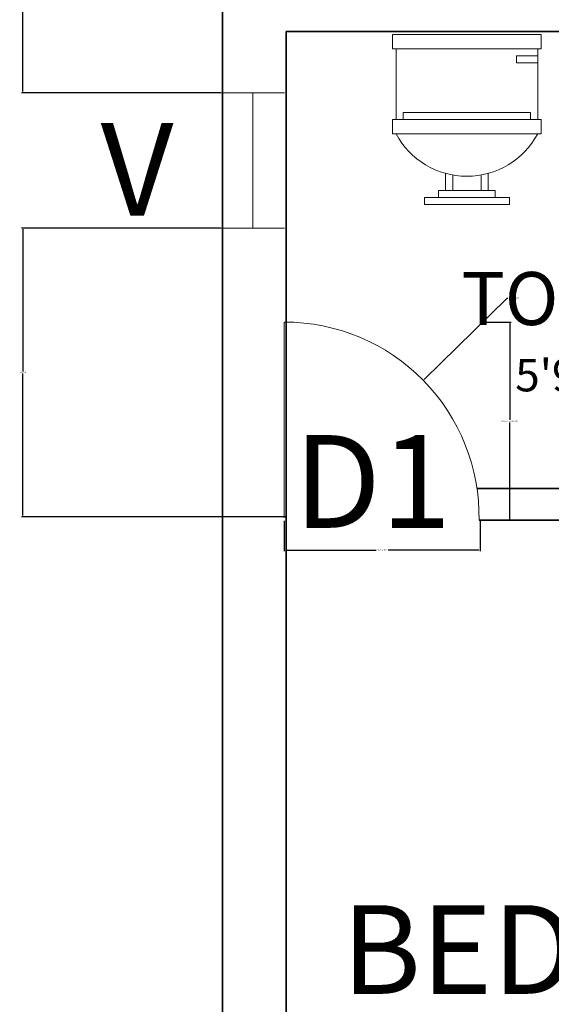
# Model space of a CAD drawing. Units: inches. Extents: x -26 to 788, y -42 to 505.
# Tile 2 of 9: x -26 to 49, y 123 to 262. Entities that reach past the tile are written whole.
import ezdxf

# ---------------------------------------------------------------- set-up
doc = ezdxf.new("R2010")
doc.units = ezdxf.units.IN
doc.header["$MEASUREMENT"] = 0
for name, color, linetype, lineweight in [('A-ANNO-DIMS', 2, 'Continuous', 18), ('A-ANNO-IDEN', 3, 'Continuous', 18), ('A-AREA-IDEN', 7, 'Continuous', 18), ('A-DOOR', 3, 'Continuous', 18), ('A-FLOR-FIXT', 9, 'Continuous', 18), ('A-GLAZ', 4, 'Continuous', 18), ('A-WALL', 7, 'Continuous', 35)]:
    doc.layers.add(name, color=color, linetype=linetype, lineweight=lineweight)
doc.styles.get("Standard").update_dxf_attribs({"font": 'arial.ttf'})
doc.dimstyles.get("Standard").update_dxf_attribs({"dimtxt": 0.18, "dimasz": 0.18, "dimexe": 0.18, "dimexo": 0.0625, "dimgap": 0.09, "dimtad": 0, "dimtih": 1, "dimtoh": 1, "dimdec": 4, "dimzin": 0, "dimdsep": 46, "dimtxsty": 'Standard', "dimcen": 0.09, "dimadec": 0, "dimazin": 0, "dimtfac": 1, "dimtdec": 4, "dimtofl": 0, "dimtmove": 0, "dimatfit": 3, "dimfxl": 1, "dimtolj": 1, "dimtzin": 0, "dimarcsym": 0})

# ---------------------------------------------------------------- blocks, each defined once
blk = doc.blocks.new('*U3')
for p, q in [((-10, 12), (-10, 22)), ((10, 21), (7, 21)), ((7, 21), (7, 20)), ((10, 22), (10, 12)), ((7, 20), (10, 20)), ((-9, 13), (9, 13)), ((-9, 12), (-9, 13)), ((9, 13), (9, 12)), ((-10.5, 12), (10.5, 12)), ((-10.5, 12), (-10.5, 10)), ((10.5, 10), (10.5, 12)), ((-10.5, 10), (10.5, 10)), ((-3, 2), (-3, 4.4065)), ((3, 4.4065), (3, 2)), ((-2, 4.1658), (-2, 2)), ((2, 2), (2, 4.1658)), ((-4, 2), (4, 2)), ((-4, 1), (-4, 2)), ((4, 2), (4, 1))]:
    blk.add_line(p, q)
for points in [[(-10.5, 22), (-10.5, 24), (10.5, 24), (10.5, 22)], [(-6, 0), (-6, 1), (6, 1), (6, 0)]]:
    blk.add_lwpolyline(points, close=True)
blk.add_arc((0, 15.3333), 11.3333, 208.0725, 331.9275)
blk = doc.blocks.new('VENT-BATH')
for p, q in [((9, 19.08), (0, 19.08)), ((4.5, 19.08), (4.5, 0)), ((9, 0), (0, 0))]:
    blk.add_line(p, q)
blk = doc.blocks.new('DOOR-BATH-A')
blk.add_line((0, 27.99), (0, 0.5))
blk.add_arc((0, 0.5), 27.49, 358.9575, 90)
blk = doc.blocks.new('*D39')
at = {"layer": 'A-ANNO-DIMS', "color": 0, "lineweight": -2, "transparency": 16777216}
for p, q in [((39.37, 219.11), (43.68, 219.11)), ((43.5, 218.93), (43.5, 205.3)), ((43.5, 191.3), (43.5, 204.93)), ((39.37, 191.12), (43.68, 191.12))]:
    blk.add_line(p, q, dxfattribs=at)
at = {"layer": 'A-ANNO-DIMS', "color": 0, "transparency": 16777216}
for points in [[(43.47, 218.93), (43.53, 218.93), (43.5, 219.11)], [(43.47, 191.3), (43.53, 191.3), (43.5, 191.12)]]:
    blk.add_solid(points, dxfattribs=at)
at = {"layer": 'Defpoints', "color": 0, "transparency": 16777216}
for p in [(39.3, 219.11), (43.5, 219.11), (39.3, 191.12)]:
    blk.add_point(p, dxfattribs=at)
at = {"layer": 'A-ANNO-DIMS', "color": 0, "transparency": 16777216, "insert": (43.5, 205.11), "char_height": 0.18, "attachment_point": 5}
blk.add_mtext('\\A1;DOOR A 27.9939 TYP.', dxfattribs=at)
blk = doc.blocks.new('*D40')
at = {"layer": 'A-ANNO-DIMS', "color": 0, "lineweight": -2, "transparency": 16777216}
for p, q in [((11.68, 191.06), (11.68, 186.74)), ((39.3, 191.06), (39.3, 186.74)), ((11.86, 186.92), (24.65, 186.92)), ((39.12, 186.92), (26.34, 186.92))]:
    blk.add_line(p, q, dxfattribs=at)
at = {"layer": 'A-ANNO-DIMS', "color": 0, "transparency": 16777216}
for points in [[(11.86, 186.95), (11.86, 186.89), (11.68, 186.92)], [(39.12, 186.95), (39.12, 186.89), (39.3, 186.92)]]:
    blk.add_solid(points, dxfattribs=at)
at = {"layer": 'Defpoints', "color": 0, "transparency": 16777216}
for p in [(11.68, 191.12), (39.3, 191.12), (39.3, 186.92)]:
    blk.add_point(p, dxfattribs=at)
at = {"layer": 'A-ANNO-DIMS', "color": 0, "transparency": 16777216, "insert": (25.49, 186.92), "char_height": 0.18, "attachment_point": 5}
blk.add_mtext('\\A1;27.6234 TYP.', dxfattribs=at)
blk = doc.blocks.new('*D60')
at = {"layer": 'A-ANNO-DIMS', "color": 0, "lineweight": -2, "transparency": 16777216}
for p, q in [((3.11, 276.89), (-25.4, 276.89)), ((-25.22, 276.71), (-25.22, 264.36)), ((-25.22, 251.64), (-25.22, 263.99)), ((2.66, 251.46), (-25.4, 251.46))]:
    blk.add_line(p, q, dxfattribs=at)
at = {"layer": 'A-ANNO-DIMS', "color": 0, "transparency": 16777216}
for points in [[(-25.25, 276.71), (-25.19, 276.71), (-25.22, 276.89)], [(-25.25, 251.64), (-25.19, 251.64), (-25.22, 251.46)]]:
    blk.add_solid(points, dxfattribs=at)
at = {"layer": 'Defpoints', "color": 0, "transparency": 16777216}
for p in [(-25.22, 276.89), (3.17, 276.89), (2.73, 251.46)]:
    blk.add_point(p, dxfattribs=at)
at = {"layer": 'A-ANNO-DIMS', "color": 0, "transparency": 16777216, "insert": (-25.22, 264.17), "char_height": 0.18, "attachment_point": 5}
blk.add_mtext('\\A1;25.4255', dxfattribs=at)
blk = doc.blocks.new('*D61')
at = {"layer": 'A-ANNO-DIMS', "color": 0, "lineweight": -2, "transparency": 16777216}
for p, q in [((2.66, 232.38), (-25.4, 232.38)), ((-25.22, 232.2), (-25.22, 212.18)), ((-25.22, 191.8), (-25.22, 211.82)), ((11.62, 191.62), (-25.4, 191.62))]:
    blk.add_line(p, q, dxfattribs=at)
at = {"layer": 'A-ANNO-DIMS', "color": 0, "transparency": 16777216}
for points in [[(-25.25, 232.2), (-25.19, 232.2), (-25.22, 232.38)], [(-25.25, 191.8), (-25.19, 191.8), (-25.22, 191.62)]]:
    blk.add_solid(points, dxfattribs=at)
at = {"layer": 'Defpoints', "color": 0, "transparency": 16777216}
for p in [(2.73, 232.38), (-25.22, 191.62), (11.68, 191.62)]:
    blk.add_point(p, dxfattribs=at)
at = {"layer": 'A-ANNO-DIMS', "color": 0, "transparency": 16777216, "insert": (-25.22, 212), "char_height": 0.18, "attachment_point": 5}
blk.add_mtext('\\A1;40.7640', dxfattribs=at)
blk = doc.blocks.new('*D66')
at = {"layer": 'A-ANNO-DIMS', "color": 0, "lineweight": -2, "transparency": 16777216}
for p, q in [((43.07, 222.44), (31.43, 211.01)), ((43.25, 222.44), (43.07, 222.44)), ((11.59, 191.62), (11.77, 191.62)), ((11.68, 191.53), (11.68, 191.71))]:
    blk.add_line(p, q, dxfattribs=at)
at = {"layer": 'A-ANNO-DIMS', "color": 0, "transparency": 16777216}
blk.add_solid([(31.41, 211.03), (31.45, 210.99), (31.3, 210.88)], dxfattribs=at)
at = {"layer": 'Defpoints', "color": 0, "transparency": 16777216}
for p in [(31.3, 210.88), (11.68, 191.62)]:
    blk.add_point(p, dxfattribs=at)
at = {"layer": 'A-ANNO-DIMS', "color": 0, "transparency": 16777216, "insert": (44.06, 222.44), "char_height": 0.18, "attachment_point": 5}
blk.add_mtext('\\A1;2X R27.4937', dxfattribs=at)

msp = doc.modelspace()

# ---------------------------------------------------------------- linework, layer by layer
at = {"layer": 'A-WALL'}
for p, q in [((2.95497, 2.11777), (2.95497, 431.11777)), ((11.95497, 2.11777), (11.95497, 260.11777)), ((11.95497, 260.11777), (76.45497, 260.11777)), ((38.88227, 195.61777), (76.45497, 195.61777)), ((11.68105, 191.61798), (11.95497, 191.61417)), ((39.17022, 191.11777), (84.24893, 191.11777))]:
    msp.add_line(p, q, dxfattribs=at)

# ---------------------------------------------------------------- block references
at = {"layer": 'A-DOOR'}
msp.add_blockref('DOOR-BATH-A', (11.681, 191.118), dxfattribs=at)
at = {"layer": 'A-FLOR-FIXT'}
msp.add_blockref('*U3', (37.4442, 235.68498), dxfattribs=at)
at = {"layer": 'A-GLAZ'}
msp.add_blockref('VENT-BATH', (2.727, 232.382), dxfattribs=at)

# ---------------------------------------------------------------- texts
at = {"layer": 'A-ANNO-IDEN'}
for s, height, p in [('V', 13.09317, (-14.23796, 234.10455)), ('D1', 13.093175, (13.0353, 190.0526))]:
    msp.add_text(s, height=height, dxfattribs=at).set_placement(p)
at = {"layer": 'A-AREA-IDEN'}
for s, height, p in [('TOILET', 7.483862, (36.68656, 218.68186)), ('5\'9"X5\'9"', 4.56659, (44.26822, 209.32026)), ('BEDROOM', 12.516013, (19.77046, 124.25891))]:
    msp.add_text(s, height=height, dxfattribs=at).set_placement(p)

# ---------------------------------------------------------------- dimensions: what is measured, and where the dimension line sits
at = {"layer": 'A-ANNO-DIMS'}
for base, p1, p2, picture, middle in [((-25.22286, 276.88608), (2.72715, 251.46056), (3.17262, 276.88608), '*D60', (-25.22285, 264.17332)), ((-25.22286, 191.61798), (2.72715, 232.38197), (11.68105, 191.61798), '*D61', (-25.22285, 211.99998))]:
    dim = msp.add_linear_dim(base=base, p1=p1, p2=p2, angle=90, dimstyle='Standard', override={"dimdec": 4, "dimlfac": 1, "dimrnd": 0, "dimzin": 0, "dimdsep": 46, "dimlunit": 2}, dxfattribs=at)
    dim.commit()
    dim.dimension.update_dxf_attribs({"geometry": picture, "text_midpoint": middle})
dim = msp.add_radius_dim(center=(11.68105, 191.61798), mpoint=(31.29821, 210.8812), text='2X <>', dimstyle='Standard', override={"dimdec": 4, "dimlfac": 1, "dimrnd": 0, "dimzin": 0, "dimdsep": 46, "dimlunit": 2}, dxfattribs=at)
dim.commit()
dim.dimension.update_dxf_attribs({"geometry": '*D66', "text_midpoint": (44.0631, 222.43914), "dimtype": 164})
dim = msp.add_linear_dim(base=(43.50355, 219.1117), p1=(39.30446, 191.11777), p2=(39.30446, 219.1117), angle=90, text='DOOR A <> TYP.', dimstyle='Standard', override={"dimdec": 4, "dimlfac": 1, "dimrnd": 0, "dimzin": 0, "dimdsep": 46, "dimlunit": 2}, dxfattribs=at)
dim.commit()
dim.dimension.update_dxf_attribs({"geometry": '*D39', "text_midpoint": (43.50355, 205.11473)})
dim = msp.add_linear_dim(base=(39.30446, 186.91868), p1=(11.68105, 191.11777), p2=(39.30446, 191.11777), text='<> TYP.', dimstyle='Standard', override={"dimdec": 4, "dimlfac": 1, "dimrnd": 0, "dimzin": 0, "dimdsep": 46, "dimlunit": 2}, dxfattribs=at)
dim.commit()
dim.dimension.update_dxf_attribs({"geometry": '*D40', "text_midpoint": (25.49276, 186.91868)})

doc.saveas('drawing.dxf')
